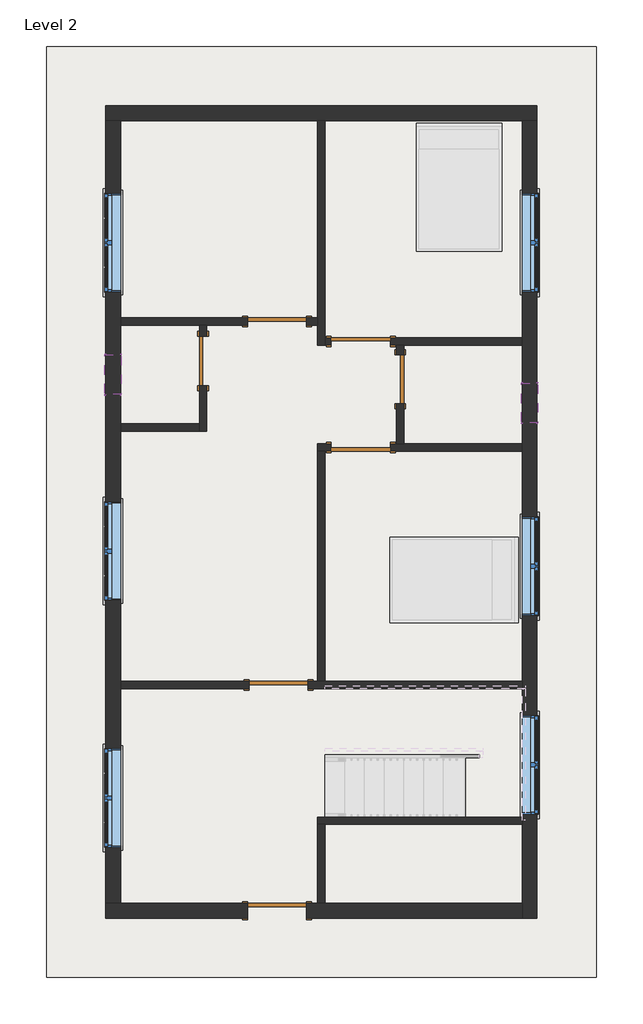
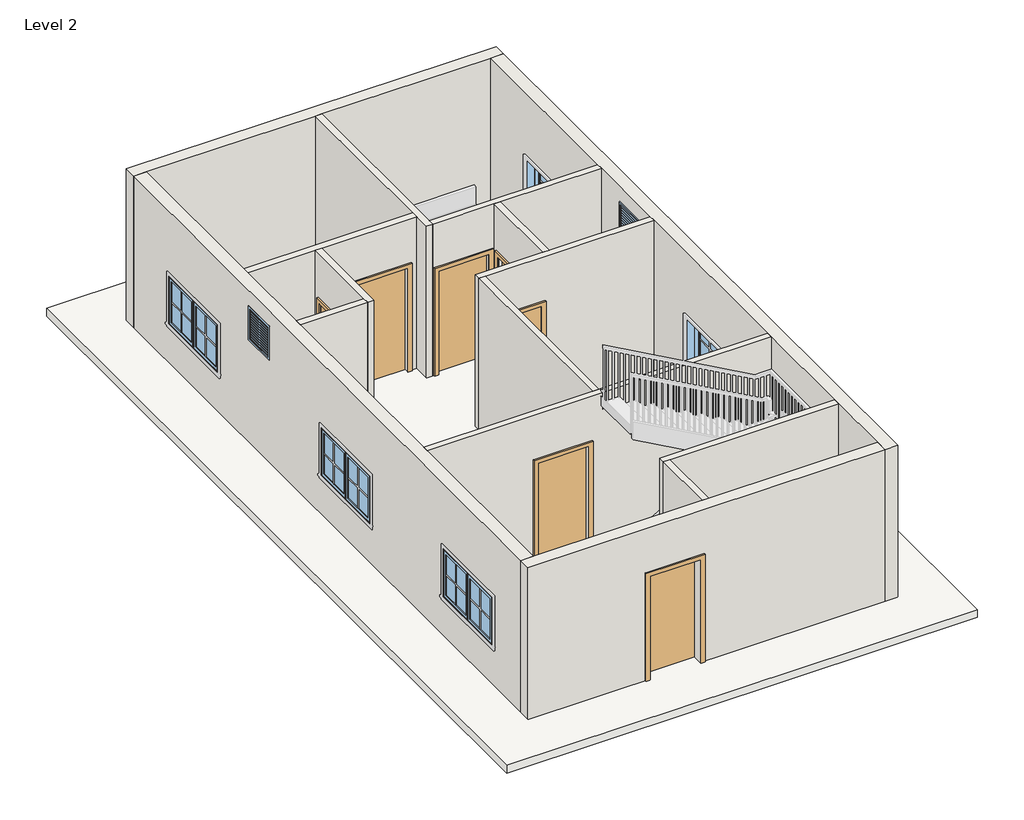
# One storey, part 1 of 3: 15 walls, 8 windows, 7 doors, 1 roof.
"""IFC4 building model written with IfcOpenShell, lengths in millimetres."""

from ifc_helpers import new_model, si_unit, frame, origin, place, context, project, spatial, polyline, outline, extrude, faceted_brep, transform, mapped, element, save
from components import door_78caadf7, door_214872d5, single_flush_door_3_e5f9f3c4, single_flush_door_3_305aa2a5, single_flush_door_3_0ca8825f, window_casement_double_win_5_c1d95f0f, window_f2d8fef0

model = new_model("IFC4")

# Units and contexts
model_context = context("Model", 3, world=origin())
ifc_project = project(units=[si_unit("LENGTHUNIT", "METRE", prefix="MILLI")], contexts=[model_context])

# Site, building, storey
site = spatial("IfcSite", under=ifc_project)
building = spatial("IfcBuilding", under=site)
storey = spatial("IfcBuildingStorey", under=building, Name="Level 2", Elevation=3048.0)

# Doors
placement = place(None, origin())
door_shape = door_78caadf7(model_context)
element("IfcDoor", 1, ObjectType="Single-Flush : 2'6\"", at=placement, inside=storey, context=model_context, shape_type="MappedRepresentation", body=[
    mapped(door_shape, transform((-35.92188, 1946.24131, 3048.0), x_axis=(0.0, 1.0, 0.0), y_axis=(-1.0, 0.0, 0.0), z_axis=(0.0, 0.0, 1.0))),
])
door_2_shape = door_214872d5(model_context)
element("IfcDoor", 2, ObjectType="Single-Flush : 2'6\"", at=placement, inside=storey, context=model_context, shape_type="MappedRepresentation", body=[
    mapped(door_2_shape, transform((-3083.92188, 2225.64131, 3048.0), x_axis=(0.0, 1.0, 0.0), y_axis=(-1.0, 0.0, 0.0), z_axis=(0.0, 0.0, 1.0))),
])
single_flush_door_3_shape = single_flush_door_3_e5f9f3c4(model_context)
element("IfcDoor", 3, ObjectType="Single-Flush : DOOR 3'", at=placement, inside=storey, context=model_context, shape_type="MappedRepresentation", body=[
    mapped(single_flush_door_3_shape, transform((-1940.92188, 2835.24131, 3048.0), x_axis=(1.0, 0.0, 0.0), y_axis=(0.0, 1.0, 0.0), z_axis=(0.0, 0.0, 1.0))),
])
element("IfcDoor", 4, ObjectType="Single-Flush : DOOR 3'", at=placement, inside=storey, context=model_context, shape_type="MappedRepresentation", body=[
    mapped(single_flush_door_3_shape, transform((-645.52188, 892.14131, 3048.0), x_axis=(-1.0, 0.0, 0.0), y_axis=(0.0, -1.0, 0.0), z_axis=(0.0, 0.0, 1.0))),
])
element("IfcDoor", 5, ObjectType="Single-Flush : DOOR 3'", at=placement, inside=storey, context=model_context, shape_type="MappedRepresentation", body=[
    mapped(single_flush_door_3_shape, transform((-1915.52188, -2778.15869, 3048.0), x_axis=(1.0, 0.0, 0.0), y_axis=(0.0, 1.0, 0.0), z_axis=(0.0, 0.0, 1.0))),
])
single_flush_door_3_2_shape = single_flush_door_3_305aa2a5(model_context)
element("IfcDoor", 6, ObjectType="Single-Flush : DOOR 3'", at=placement, inside=storey, context=model_context, shape_type="MappedRepresentation", body=[
    mapped(single_flush_door_3_2_shape, transform((-645.52188, 2530.44131, 3048.0), x_axis=(-1.0, 0.0, 0.0), y_axis=(0.0, -1.0, 0.0), z_axis=(0.0, 0.0, 1.0))),
])
single_flush_door_3_3_shape = single_flush_door_3_0ca8825f(model_context)
element("IfcDoor", 7, ObjectType="Single-Flush : DOOR 3'", at=placement, inside=storey, context=model_context, shape_type="MappedRepresentation", body=[
    mapped(single_flush_door_3_3_shape, transform((-1940.92188, -6264.30869, 3048.0), x_axis=(1.0, 0.0, 0.0), y_axis=(0.0, 1.0, 0.0), z_axis=(0.0, 0.0, 1.0))),
])

# Roof
element("IfcRoof", 8, ObjectType="ROOF 6\"", at=placement, inside=storey, context=model_context, shape_type="SweptSolid", body=[
    extrude(outline(polyline([(-5503.27188, 7083.39131), (2993.02812, 7083.39131), (2993.02812, -7293.00869), (-5503.27188, -7293.00869), (-5503.27188, 7083.39131)])), frame((0.0, 0.0, 3048.0), z_axis=(0.0, 0.0, 1.0), x_axis=(1.0, 0.0, 0.0)), (0.0, 0.0, 1.0), 152.4),
])

# Walls
element("IfcWall", 9, ObjectType="WALL 4.5'", at=placement, inside=storey, context=model_context, shape_type="Brep", body=[
    faceted_brep([(-1312.27188, 5940.39131, 3048.0), (-1312.27188, 2892.39131, 3048.0), (-1312.27188, 2778.09131, 3048.0), (-1312.27188, 2473.29131, 3048.0), (-1312.27188, 2473.29131, 6096.0), (-1312.27188, 2778.09131, 6096.0), (-1312.27188, 2892.39131, 6096.0), (-1312.27188, 5940.39131, 6096.0), (-1197.97188, 5940.39131, 3048.0), (-1197.97188, 5940.39131, 6096.0), (-1197.97188, 2587.59131, 6096.0), (-1197.97188, 2473.29131, 6096.0), (-1197.97188, 2473.29131, 3048.0), (-1197.97188, 2587.59131, 3048.0)], [[[0, 1, 2, 3, 4, 5, 6, 7]], [[8, 9, 10, 11, 12, 13]], [[3, 2, 1, 0, 8, 13, 12]], [[0, 7, 9, 8]], [[4, 3, 12, 11]], [[7, 6, 5, 4, 11, 10, 9]]]),
])
element("IfcWall", 10, ObjectType="WALL 4.5'", at=placement, inside=storey, context=model_context, shape_type="Brep", body=[
    faceted_brep([(-1197.97188, 2473.29131, 3048.0), (-1102.72188, 2473.29131, 3048.0), (-1102.72188, 2473.29131, 5181.6), (-188.32188, 2473.29131, 5181.6), (-188.32188, 2473.29131, 3048.0), (-93.07188, 2473.29131, 3048.0), (21.22812, 2473.29131, 3048.0), (1850.02812, 2473.29131, 3048.0), (1850.02812, 2473.29131, 6096.0), (21.22812, 2473.29131, 6096.0), (-93.07188, 2473.29131, 6096.0), (-1197.97188, 2473.29131, 6096.0), (-1102.72188, 2587.59131, 5181.6), (-1102.72188, 2587.59131, 3048.0), (-1197.97188, 2587.59131, 3048.0), (-1197.97188, 2587.59131, 6096.0), (1850.02812, 2587.59131, 6096.0), (1850.02812, 2587.59131, 3048.0), (-188.32188, 2587.59131, 3048.0), (-188.32188, 2587.59131, 5181.6)], [[[0, 1, 2, 3, 4, 5, 6, 7, 8, 9, 10, 11]], [[12, 13, 14, 15, 16, 17, 18, 19]], [[18, 17, 7, 6, 5, 4]], [[14, 13, 1, 0]], [[0, 11, 15, 14]], [[8, 7, 17, 16]], [[2, 1, 13, 12]], [[3, 2, 12, 19]], [[4, 3, 19, 18]], [[11, 10, 9, 8, 16, 15]]]),
])
element("IfcWall", 11, ObjectType="WALL 4.5'", at=placement, inside=storey, context=model_context, shape_type="Brep", body=[
    faceted_brep([(-1312.27188, 2892.39131, 3048.0), (-1483.72188, 2892.39131, 3048.0), (-1483.72188, 2892.39131, 5181.6), (-2398.12188, 2892.39131, 5181.6), (-2398.12188, 2892.39131, 3048.0), (-4360.27188, 2892.39131, 3048.0), (-4360.27188, 2892.39131, 6096.0), (-1312.27188, 2892.39131, 6096.0), (-1483.72188, 2778.09131, 5181.6), (-1483.72188, 2778.09131, 3048.0), (-1312.27188, 2778.09131, 3048.0), (-1312.27188, 2778.09131, 6096.0), (-3026.77188, 2778.09131, 6096.0), (-3141.07188, 2778.09131, 6096.0), (-4360.27188, 2778.09131, 6096.0), (-4360.27188, 2778.09131, 3048.0), (-3141.07188, 2778.09131, 3048.0), (-3026.77188, 2778.09131, 3048.0), (-2398.12188, 2778.09131, 3048.0), (-2398.12188, 2778.09131, 5181.6)], [[[0, 1, 2, 3, 4, 5, 6, 7]], [[8, 9, 10, 11, 12, 13, 14, 15, 16, 17, 18, 19]], [[10, 9, 1, 0]], [[18, 17, 16, 15, 5, 4]], [[6, 5, 15, 14]], [[0, 7, 11, 10]], [[2, 1, 9, 8]], [[3, 2, 8, 19]], [[4, 3, 19, 18]], [[7, 6, 14, 13, 12, 11]]]),
])
element("IfcWall", 12, ObjectType="WALL 4.5'", at=placement, inside=storey, context=model_context, shape_type="Brep", body=[
    faceted_brep([(-3141.07188, 2778.09131, 3048.0), (-3141.07188, 2606.64131, 3048.0), (-3141.07188, 2606.64131, 5181.6), (-3141.07188, 1844.64131, 5181.6), (-3141.07188, 1844.64131, 3048.0), (-3141.07188, 1254.09131, 3048.0), (-3141.07188, 1139.79131, 3048.0), (-3141.07188, 1139.79131, 6096.0), (-3141.07188, 1254.09131, 6096.0), (-3141.07188, 2778.09131, 6096.0), (-3026.77188, 2606.64131, 5181.6), (-3026.77188, 2606.64131, 3048.0), (-3026.77188, 2778.09131, 3048.0), (-3026.77188, 2778.09131, 6096.0), (-3026.77188, 1139.79131, 6096.0), (-3026.77188, 1139.79131, 3048.0), (-3026.77188, 1844.64131, 3048.0), (-3026.77188, 1844.64131, 5181.6)], [[[0, 1, 2, 3, 4, 5, 6, 7, 8, 9]], [[10, 11, 12, 13, 14, 15, 16, 17]], [[16, 15, 6, 5, 4]], [[12, 11, 1, 0]], [[0, 9, 13, 12]], [[7, 6, 15, 14]], [[2, 1, 11, 10]], [[3, 2, 10, 17]], [[4, 3, 17, 16]], [[9, 8, 7, 14, 13]]]),
])
element("IfcWall", 13, ObjectType="WALL 4.5'", at=placement, inside=storey, context=model_context, shape_type="SweptSolid", body=[
    extrude(outline(polyline([(-4360.27188, 1254.09131), (-3141.07188, 1254.09131), (-3141.07188, 1139.79131), (-4360.27188, 1139.79131), (-4360.27188, 1254.09131)])), frame((0.0, 0.0, 3048.0), z_axis=(0.0, 0.0, 1.0), x_axis=(1.0, 0.0, 0.0)), (0.0, 0.0, 1.0), 3048.0),
])
element("IfcWall", 14, ObjectType="WALL 4.5'", at=placement, inside=storey, context=model_context, shape_type="SweptSolid", body=[
    extrude(outline(polyline([(2473.29131, 3048.0), (2327.24131, 3048.0), (2327.24131, 5181.6), (1565.24131, 5181.6), (1565.24131, 3048.0), (949.29131, 3048.0), (949.29131, 6096.0), (2473.29131, 6096.0), (2473.29131, 3048.0)])), frame((-93.07188, 0.0, 0.0), z_axis=(1.0, 0.0, 0.0), x_axis=(0.0, 1.0, 0.0)), (0.0, 0.0, 1.0), 114.3),
])
element("IfcWall", 15, ObjectType="WALL 4.5'", at=placement, inside=storey, context=model_context, shape_type="Brep", body=[
    faceted_brep([(-1102.72188, 949.29131, 5181.6), (-1102.72188, 949.29131, 3048.0), (-1312.27188, 949.29131, 3048.0), (-1312.27188, 949.29131, 6096.0), (-93.07188, 949.29131, 6096.0), (21.22812, 949.29131, 6096.0), (1850.02812, 949.29131, 6096.0), (1850.02812, 949.29131, 3048.0), (21.22812, 949.29131, 3048.0), (-93.07188, 949.29131, 3048.0), (-188.32188, 949.29131, 3048.0), (-188.32188, 949.29131, 5181.6), (-1312.27188, 834.99131, 3048.0), (-1197.97188, 834.99131, 3048.0), (-1102.72188, 834.99131, 3048.0), (-1102.72188, 834.99131, 5181.6), (-188.32188, 834.99131, 5181.6), (-188.32188, 834.99131, 3048.0), (1850.02812, 834.99131, 3048.0), (1850.02812, 834.99131, 6096.0), (-1197.97188, 834.99131, 6096.0), (-1312.27188, 834.99131, 6096.0)], [[[0, 1, 2, 3, 4, 5, 6, 7, 8, 9, 10, 11]], [[12, 13, 14, 15, 16, 17, 18, 19, 20, 21]], [[2, 1, 14, 13, 12]], [[10, 9, 8, 7, 18, 17]], [[7, 6, 19, 18]], [[3, 2, 12, 21]], [[15, 14, 1, 0]], [[16, 15, 0, 11]], [[17, 16, 11, 10]], [[6, 5, 4, 3, 21, 20, 19]]]),
])
element("IfcWall", 16, ObjectType="WALL 4.5'", at=placement, inside=storey, context=model_context, shape_type="SweptSolid", body=[
    extrude(outline(polyline([(-1312.27188, -2721.00869), (-1312.27188, 834.99131), (-1197.97188, 834.99131), (-1197.97188, -2721.00869), (-1312.27188, -2721.00869)])), frame((0.0, 0.0, 3048.0), z_axis=(0.0, 0.0, 1.0), x_axis=(1.0, 0.0, 0.0)), (0.0, 0.0, 1.0), 3048.0),
])
element("IfcWall", 17, ObjectType="WALL 4.5'", at=placement, inside=storey, context=model_context, shape_type="Brep", body=[
    faceted_brep([(1850.02812, -2721.00869, 3048.0), (-1197.97188, -2721.00869, 3048.0), (-1312.27188, -2721.00869, 3048.0), (-1458.32188, -2721.00869, 3048.0), (-1458.32188, -2721.00869, 5181.6), (-2372.72188, -2721.00869, 5181.6), (-2372.72188, -2721.00869, 3048.0), (-4360.27188, -2721.00869, 3048.0), (-4360.27188, -2721.00869, 6096.0), (-1312.27188, -2721.00869, 6096.0), (-1197.97188, -2721.00869, 6096.0), (1850.02812, -2721.00869, 6096.0), (-1458.32188, -2835.30869, 5181.6), (-1458.32188, -2835.30869, 3048.0), (1850.02812, -2835.30869, 3048.0), (1850.02812, -2835.30869, 6096.0), (-4360.27188, -2835.30869, 6096.0), (-4360.27188, -2835.30869, 3048.0), (-2372.72188, -2835.30869, 3048.0), (-2372.72188, -2835.30869, 5181.6)], [[[0, 1, 2, 3, 4, 5, 6, 7, 8, 9, 10, 11]], [[12, 13, 14, 15, 16, 17, 18, 19]], [[18, 17, 7, 6]], [[14, 13, 3, 2, 1, 0]], [[0, 11, 15, 14]], [[8, 7, 17, 16]], [[4, 3, 13, 12]], [[5, 4, 12, 19]], [[6, 5, 19, 18]], [[11, 10, 9, 8, 16, 15]]]),
])
element("IfcWall", 18, ObjectType="WALL 4.5'", at=placement, inside=storey, context=model_context, shape_type="Brep", body=[
    faceted_brep([(1850.02812, -4816.50869, 3048.0), (-1312.27188, -4816.50869, 3048.0), (-1312.27188, -4816.50869, 6096.0), (1850.02812, -4816.50869, 6096.0), (1850.02812, -4930.80869, 3048.0), (1850.02812, -4930.80869, 6096.0), (-1197.97188, -4930.80869, 6096.0), (-1312.27188, -4930.80869, 6096.0), (-1312.27188, -4930.80869, 3048.0), (-1197.97188, -4930.80869, 3048.0)], [[[0, 1, 2, 3]], [[4, 5, 6, 7, 8, 9]], [[1, 0, 4, 9, 8]], [[0, 3, 5, 4]], [[2, 1, 8, 7]], [[3, 2, 7, 6, 5]]]),
])
element("IfcWall", 19, ObjectType="WALL 4.5'", at=placement, inside=storey, context=model_context, shape_type="SweptSolid", body=[
    extrude(outline(polyline([(-1312.27188, -6150.00869), (-1312.27188, -4930.80869), (-1197.97188, -4930.80869), (-1197.97188, -6150.00869), (-1312.27188, -6150.00869)])), frame((0.0, 0.0, 3048.0), z_axis=(0.0, 0.0, 1.0), x_axis=(1.0, 0.0, 0.0)), (0.0, 0.0, 1.0), 3048.0),
])
element("IfcWall", 20, ObjectType="WALL 9\"", at=placement, inside=storey, context=model_context, shape_type="Brep", body=[
    faceted_brep([(-4588.87188, 5940.39131, 3048.0), (-4360.27188, 5940.39131, 3048.0), (-1312.27188, 5940.39131, 3048.0), (-1197.97188, 5940.39131, 3048.0), (1850.02812, 5940.39131, 3048.0), (2078.62812, 5940.39131, 3048.0), (2078.62812, 5940.39131, 6096.0), (1850.02812, 5940.39131, 6096.0), (-1197.97188, 5940.39131, 6096.0), (-1312.27188, 5940.39131, 6096.0), (-4360.27188, 5940.39131, 6096.0), (-4588.87188, 5940.39131, 6096.0), (-4588.87188, 6168.99131, 3048.0), (-4588.87188, 6168.99131, 6096.0), (2078.62812, 6168.99131, 6096.0), (2078.62812, 6168.99131, 3048.0)], [[[0, 1, 2, 3, 4, 5, 6, 7, 8, 9, 10, 11]], [[12, 13, 14, 15]], [[5, 4, 3, 2, 1, 0, 12, 15]], [[6, 5, 15, 14]], [[0, 11, 13, 12]], [[11, 10, 9, 8, 7, 6, 14, 13]]]),
])
element("IfcWall", 21, ObjectType="WALL 9\"", at=placement, inside=storey, context=model_context, shape_type="Brep", body=[
    faceted_brep([(1850.02812, 5940.39131, 3048.0), (1850.02812, 2587.59131, 3048.0), (1850.02812, 2473.29131, 3048.0), (1850.02812, 949.29131, 3048.0), (1850.02812, 834.99131, 3048.0), (1850.02812, -2721.00869, 3048.0), (1850.02812, -2835.30869, 3048.0), (1850.02812, -4816.50869, 3048.0), (1850.02812, -4930.80869, 3048.0), (1850.02812, -6150.00869, 3048.0), (1850.02812, -6378.60869, 3048.0), (1850.02812, -6378.60869, 6096.0), (1850.02812, -6150.00869, 6096.0), (1850.02812, -4930.80869, 6096.0), (1850.02812, -4816.50869, 6096.0), (1850.02812, -2835.30869, 6096.0), (1850.02812, -2721.00869, 6096.0), (1850.02812, 834.99131, 6096.0), (1850.02812, 949.29131, 6096.0), (1850.02812, 2473.29131, 6096.0), (1850.02812, 2587.59131, 6096.0), (1850.02812, 5940.39131, 6096.0), (1850.02812, -4772.05869, 4876.8), (1850.02812, -4772.05869, 3962.4), (1850.02812, -3248.05869, 3962.4), (1850.02812, -3248.05869, 4876.8), (1850.02812, 3292.44131, 4876.8), (1850.02812, 3292.44131, 3962.4), (1850.02812, 4816.44131, 3962.4), (1850.02812, 4816.44131, 4876.8), (1850.02812, -1705.00869, 4876.8), (1850.02812, -1705.00869, 3962.4), (1850.02812, -181.00869, 3962.4), (1850.02812, -181.00869, 4876.8), (1850.02812, 1273.14131, 5791.2), (1850.02812, 1273.14131, 5181.6), (1850.02812, 1882.74131, 5181.6), (1850.02812, 1882.74131, 5791.2), (2078.62812, 5940.39131, 3048.0), (2078.62812, 5940.39131, 6096.0), (2078.62812, -6378.60869, 6096.0), (2078.62812, -6378.60869, 3048.0), (2078.62812, -4772.05869, 4876.8), (2078.62812, -3248.05869, 4876.8), (2078.62812, -3248.05869, 3962.4), (2078.62812, -4772.05869, 3962.4), (2078.62812, 3292.44131, 4876.8), (2078.62812, 4816.44131, 4876.8), (2078.62812, 4816.44131, 3962.4), (2078.62812, 3292.44131, 3962.4), (2078.62812, -1705.00869, 4876.8), (2078.62812, -181.00869, 4876.8), (2078.62812, -181.00869, 3962.4), (2078.62812, -1705.00869, 3962.4), (2078.62812, 1273.14131, 5791.2), (2078.62812, 1882.74131, 5791.2), (2078.62812, 1882.74131, 5181.6), (2078.62812, 1273.14131, 5181.6)], [[[0, 1, 2, 3, 4, 5, 6, 7, 8, 9, 10, 11, 12, 13, 14, 15, 16, 17, 18, 19, 20, 21], [22, 23, 24, 25], [26, 27, 28, 29], [30, 31, 32, 33], [34, 35, 36, 37]], [[38, 39, 40, 41], [42, 43, 44, 45], [46, 47, 48, 49], [50, 51, 52, 53], [54, 55, 56, 57]], [[10, 9, 8, 7, 6, 5, 4, 3, 2, 1, 0, 38, 41]], [[0, 21, 39, 38]], [[11, 10, 41, 40]], [[23, 22, 42, 45]], [[24, 23, 45, 44]], [[25, 24, 44, 43]], [[22, 25, 43, 42]], [[27, 26, 46, 49]], [[28, 27, 49, 48]], [[29, 28, 48, 47]], [[26, 29, 47, 46]], [[31, 30, 50, 53]], [[32, 31, 53, 52]], [[33, 32, 52, 51]], [[30, 33, 51, 50]], [[35, 34, 54, 57]], [[36, 35, 57, 56]], [[37, 36, 56, 55]], [[34, 37, 55, 54]], [[21, 20, 19, 18, 17, 16, 15, 14, 13, 12, 11, 40, 39]]]),
])
element("IfcWall", 22, ObjectType="WALL 9\"", at=placement, inside=storey, context=model_context, shape_type="Brep", body=[
    faceted_brep([(1850.02812, -6150.00869, 3048.0), (-1197.97188, -6150.00869, 3048.0), (-1312.27188, -6150.00869, 3048.0), (-1483.72188, -6150.00869, 3048.0), (-1483.72188, -6150.00869, 5181.6), (-2398.12188, -6150.00869, 5181.6), (-2398.12188, -6150.00869, 3048.0), (-4360.27188, -6150.00869, 3048.0), (-4588.87188, -6150.00869, 3048.0), (-4588.87188, -6150.00869, 6096.0), (-4360.27188, -6150.00869, 6096.0), (-1312.27188, -6150.00869, 6096.0), (-1197.97188, -6150.00869, 6096.0), (1850.02812, -6150.00869, 6096.0), (-1483.72188, -6378.60869, 5181.6), (-1483.72188, -6378.60869, 3048.0), (1850.02812, -6378.60869, 3048.0), (1850.02812, -6378.60869, 6096.0), (-4588.87188, -6378.60869, 6096.0), (-4588.87188, -6378.60869, 3048.0), (-2398.12188, -6378.60869, 3048.0), (-2398.12188, -6378.60869, 5181.6)], [[[0, 1, 2, 3, 4, 5, 6, 7, 8, 9, 10, 11, 12, 13]], [[14, 15, 16, 17, 18, 19, 20, 21]], [[20, 19, 8, 7, 6]], [[16, 15, 3, 2, 1, 0]], [[0, 13, 17, 16]], [[9, 8, 19, 18]], [[4, 3, 15, 14]], [[5, 4, 14, 21]], [[6, 5, 21, 20]], [[13, 12, 11, 10, 9, 18, 17]]]),
])
element("IfcWall", 23, ObjectType="WALL 9\"", at=placement, inside=storey, context=model_context, shape_type="Brep", body=[
    faceted_brep([(-4360.27188, -6150.00869, 3048.0), (-4360.27188, -2835.30869, 3048.0), (-4360.27188, -2721.00869, 3048.0), (-4360.27188, 1139.79131, 3048.0), (-4360.27188, 1254.09131, 3048.0), (-4360.27188, 2778.09131, 3048.0), (-4360.27188, 2892.39131, 3048.0), (-4360.27188, 5940.39131, 3048.0), (-4360.27188, 5940.39131, 6096.0), (-4360.27188, 2892.39131, 6096.0), (-4360.27188, 2778.09131, 6096.0), (-4360.27188, 1254.09131, 6096.0), (-4360.27188, 1139.79131, 6096.0), (-4360.27188, -2721.00869, 6096.0), (-4360.27188, -2835.30869, 6096.0), (-4360.27188, -6150.00869, 6096.0), (-4360.27188, 4816.44131, 4876.8), (-4360.27188, 4816.44131, 3962.4), (-4360.27188, 3292.44131, 3962.4), (-4360.27188, 3292.44131, 4876.8), (-4360.27188, 53.94131, 4876.8), (-4360.27188, 53.94131, 3962.4), (-4360.27188, -1470.05869, 3962.4), (-4360.27188, -1470.05869, 4876.8), (-4360.27188, -3759.23369, 4876.8), (-4360.27188, -3759.23369, 3962.4), (-4360.27188, -5283.23369, 3962.4), (-4360.27188, -5283.23369, 4876.8), (-4360.27188, 1711.29131, 5791.2), (-4360.27188, 2320.89131, 5791.2), (-4360.27188, 2320.89131, 5181.6), (-4360.27188, 1711.29131, 5181.6), (-4588.87188, -6150.00869, 3048.0), (-4588.87188, -6150.00869, 6096.0), (-4588.87188, 5940.39131, 6096.0), (-4588.87188, 5940.39131, 3048.0), (-4588.87188, 4816.44131, 4876.8), (-4588.87188, 3292.44131, 4876.8), (-4588.87188, 3292.44131, 3962.4), (-4588.87188, 4816.44131, 3962.4), (-4588.87188, 53.94131, 4876.8), (-4588.87188, -1470.05869, 4876.8), (-4588.87188, -1470.05869, 3962.4), (-4588.87188, 53.94131, 3962.4), (-4588.87188, -3759.23369, 4876.8), (-4588.87188, -5283.23369, 4876.8), (-4588.87188, -5283.23369, 3962.4), (-4588.87188, -3759.23369, 3962.4), (-4588.87188, 1711.29131, 5791.2), (-4588.87188, 1711.29131, 5181.6), (-4588.87188, 2320.89131, 5181.6), (-4588.87188, 2320.89131, 5791.2)], [[[0, 1, 2, 3, 4, 5, 6, 7, 8, 9, 10, 11, 12, 13, 14, 15], [16, 17, 18, 19], [20, 21, 22, 23], [24, 25, 26, 27], [28, 29, 30, 31]], [[32, 33, 34, 35], [36, 37, 38, 39], [40, 41, 42, 43], [44, 45, 46, 47], [48, 49, 50, 51]], [[7, 6, 5, 4, 3, 2, 1, 0, 32, 35]], [[8, 7, 35, 34]], [[0, 15, 33, 32]], [[17, 16, 36, 39]], [[18, 17, 39, 38]], [[19, 18, 38, 37]], [[16, 19, 37, 36]], [[21, 20, 40, 43]], [[22, 21, 43, 42]], [[23, 22, 42, 41]], [[20, 23, 41, 40]], [[25, 24, 44, 47]], [[26, 25, 47, 46]], [[27, 26, 46, 45]], [[24, 27, 45, 44]], [[49, 48, 28, 31]], [[50, 49, 31, 30]], [[51, 50, 30, 29]], [[48, 51, 29, 28]], [[15, 14, 13, 12, 11, 10, 9, 8, 34, 33]]]),
])

# Windows
window_casement_double_win_5_shape = window_casement_double_win_5_c1d95f0f(model_context)
element("IfcWindow", 24, ObjectType="Window-Casement-Double : WIN 5'", at=placement, inside=storey, context=model_context, shape_type="MappedRepresentation", body=[
    mapped(window_casement_double_win_5_shape, transform((-4474.57188, 4054.44131, 3048.0), x_axis=(0.0, 1.0, 0.0), y_axis=(-1.0, 0.0, 0.0), z_axis=(0.0, 0.0, 1.0))),
])
element("IfcWindow", 25, ObjectType="Window-Casement-Double : WIN 5'", at=placement, inside=storey, context=model_context, shape_type="MappedRepresentation", body=[
    mapped(window_casement_double_win_5_shape, transform((-4474.57188, -708.05869, 3048.0), x_axis=(0.0, 1.0, 0.0), y_axis=(-1.0, 0.0, 0.0), z_axis=(0.0, 0.0, 1.0))),
])
element("IfcWindow", 26, ObjectType="Window-Casement-Double : WIN 5'", at=placement, inside=storey, context=model_context, shape_type="MappedRepresentation", body=[
    mapped(window_casement_double_win_5_shape, transform((-4474.57188, -4521.23369, 3048.0), x_axis=(0.0, 1.0, 0.0), y_axis=(-1.0, 0.0, 0.0), z_axis=(0.0, 0.0, 1.0))),
])
element("IfcWindow", 27, ObjectType="Window-Casement-Double : WIN 5'", at=placement, inside=storey, context=model_context, shape_type="MappedRepresentation", body=[
    mapped(window_casement_double_win_5_shape, transform((1964.32812, -4010.05869, 3048.0), x_axis=(0.0, -1.0, 0.0), y_axis=(1.0, 0.0, 0.0), z_axis=(0.0, 0.0, 1.0))),
])
element("IfcWindow", 28, ObjectType="Window-Casement-Double : WIN 5'", at=placement, inside=storey, context=model_context, shape_type="MappedRepresentation", body=[
    mapped(window_casement_double_win_5_shape, transform((1964.32812, 4054.44131, 3048.0), x_axis=(0.0, -1.0, 0.0), y_axis=(1.0, 0.0, 0.0), z_axis=(0.0, 0.0, 1.0))),
])
element("IfcWindow", 29, ObjectType="Window-Casement-Double : WIN 5'", at=placement, inside=storey, context=model_context, shape_type="MappedRepresentation", body=[
    mapped(window_casement_double_win_5_shape, transform((1964.32812, -943.00869, 3048.0), x_axis=(0.0, -1.0, 0.0), y_axis=(1.0, 0.0, 0.0), z_axis=(0.0, 0.0, 1.0))),
])
window_shape = window_f2d8fef0(model_context)
element("IfcWindow", 30, ObjectType="Window-Louvers : 24\" x 24\"", at=placement, inside=storey, context=model_context, shape_type="MappedRepresentation", body=[
    mapped(window_shape, transform((1957.97812, 1577.94131, 4267.2), x_axis=(0.0, 1.0, 0.0), y_axis=(-1.0, 0.0, 0.0), z_axis=(0.0, 0.0, 1.0))),
])
element("IfcWindow", 31, ObjectType="Window-Louvers : 24\" x 24\"", at=placement, inside=storey, context=model_context, shape_type="MappedRepresentation", body=[
    mapped(window_shape, transform((-4480.92188, 2016.09131, 4267.2), x_axis=(0.0, 1.0, 0.0), y_axis=(-1.0, 0.0, 0.0), z_axis=(0.0, 0.0, 1.0))),
])

save(model, "model.ifc")

# Revit data of these elements
# Type "Single-Flush : 2'6\""
#   Type Mark = "9"
#   Construction Type Id = "MDOOR"
#   Assembly Code = "C1020"
#   Analytic Construction = "Metal"
#   Thickness = 0' - 2"
#   Heat Transfer Coefficient (U) = 0.651978 BTU/(h·ft²·°F)
#   Height = 7' - 0"
#   Trim Projection Ext = 0' - 1"
#   Trim Projection Int = 0' - 1"
#   Trim Width = 0' - 3"
#   Width = 2' - 6"
#   Define Thermal Properties by = 1
#   Door Material = Door - Panel
#   Frame Material = Door - Frame
#   Visual Light Transmittance = 0
#   Solar Heat Gain Coefficient = 0
#   Function = (empty or 0)
#   Wall Closure = (empty or 0)
# Type "Single-Flush : DOOR 3'"
#   Type Mark = "8"
#   Construction Type Id = "MDOOR"
#   Assembly Code = "C1020"
#   Analytic Construction = "Metal"
#   Thickness = 0' - 2"
#   Heat Transfer Coefficient (U) = 0.651978 BTU/(h·ft²·°F)
#   Height = 7' - 0"
#   Trim Projection Ext = 0' - 1"
#   Trim Projection Int = 0' - 1"
#   Trim Width = 0' - 3"
#   Width = 3' - 0"
#   Define Thermal Properties by = 1
#   Door Material = Door - Panel
#   Frame Material = Door - Frame
#   Visual Light Transmittance = 0
#   Solar Heat Gain Coefficient = 0
#   Function = (empty or 0)
#   Wall Closure = (empty or 0)
# Type "ROOF 6\""
#   Assembly Code = "B1020"
#   Layers, outside or top first: 0' - 6" no material (function 1)
# Type "WALL 4.5'"
#   Assembly Code = "B2010"
#   Layers, outside or top first: 0' - 4 1/2" no material (function 1)
# Type "WALL 9\""
#   Assembly Code = "B2010"
#   Layers, outside or top first: 0' - 9" no material (function 1)
# Type "Window-Casement-Double : WIN 5'"
#   Type Mark = "18"
#   Fire Rating = "0.5h"
#   Assembly Code = "B2020100"
#   Analytic Construction = "Double glazing - domestic"
#   Frame Extension [instance default] = 0' - 0 1/4"
#   Window Inset [instance default] = 0' - 0"
#   Wall Thickness [instance default] = 0' - 6"
#   Interior Wall Closure [instance default] = 0' - 2 1/4"
#   Half Width = 2' - 6"
#   Visual Light Transmittance = 0.81
#   Thermal Resistance (R) = 1.8146 (h·ft²·°F)/BTU
#   Solar Heat Gain Coefficient = 0.76
#   Rough Width = 5' - 0 1/2"
#   Rough Height = 3' - 0 1/2"
#   Height = 3' - 0"
#   Heat Transfer Coefficient (U) = 0.5511 BTU/(h·ft²·°F)
#   Exterior Wall Closure [instance default] = 0' - 1 1/4"
#   Extension Jamb [instance default] = 0' - 2 1/4"
#   Default Sill Height = 3' - 0"
#   Width = 5' - 0"
#   Muntin Visibility = yes
#   Interior Trim Visibility [instance default] = yes
#   Exterior Trim Visibility [instance default] = yes
#   Extension Jamb Visibility [instance default] = yes
#   Interior Trim Material = Wood - Stained
#   Muntin Pattern = Muntin Pattern_2x2 : Muntin Pattern_2x2
#   Interior Trim = Trim-Window-Interior-Flat : Picture Frame
#   Interior Frame Material = Wood - Stained
#   Glass Panel Material = Glass
#   Exterior Trim Material = Clad - White
#   Exterior Trim = Trim-Window-Exterior-Flat : with Sill
#   Exterior Frame Material = Clad - White
#   Wall Closure = (empty or 0)
# Type "Window-Louvers : 24\" x 24\""
#   Type Mark = "19"
#   Construction Type Id = "GSP4R"
#   Assembly Code = "B20"
#   Analytic Construction = "1/8 in Pilkington single glazing"
#   Visual Light Transmittance = 0.9
#   Thermal Resistance (R) = 1.53941 (h·ft²·°F)/BTU
#   Solar Heat Gain Coefficient = 0.78
#   Max Height = 1' - 11.74264"
#   Height = 2' - 0"
#   Heat Transfer Coefficient (U) = 0.6496 BTU/(h·ft²·°F)
#   Blade Width [instance default] = 1' - 10 1/2"
#   Blade Vertical Thickness = 0' - 0.35355"
#   Blade Thickness = 0' - 0 1/4"
#   Blade Spacing = 0' - 1 1/2"
#   Blade Height = 0' - 1.85355"
#   Blade Depth = 0' - 3"
#   Blade Angle = 45.00°
#   Default Sill Height = 3' - 0"
#   Trim Projection_Exterior = 0' - 0 1/2"
#   Trim Projection_Interior = 0' - 0 1/2"
#   Trim Width_Exterior = 0' - 1 1/2"
#   Trim Width_Interior = 0' - 1 1/2"
#   Width = 2' - 0"
#   Max Blade Count = 12
#   Define Thermal Properties by = 1
#   Blade Count = 12
#   Frame Material = Birch
#   Louver Material = Birch
#   Trim Exterior Material = Birch
#   Trim Interior Material = Birch
#   Wall Closure = (empty or 0)
# Elements 1, 2 (IfcDoor, "Single-Flush : 2'6\"")
#   Phase Created = New Construction
#   Materials on its faces: "Door - Frame", "Door - Panel"
# Elements 3, 4, 5, 6, 7 (IfcDoor, "Single-Flush : DOOR 3'")
#   Phase Created = New Construction
#   Materials on its faces: "Door - Frame", "Door - Panel"
# Element 8 (IfcRoof, "ROOF 6\"")
#   built-in parameter 1001705 = 10.5 (stored number, unit not read)
#   built-in parameter 1001710 = 33615
#   Phase Created = New Construction
#   Materials on its faces: "Parking Stripe", "Default Roof", "Wood - Stained"
# Elements 9, 10, 11, 12, 13, 14, 15, 16, 17, 18, 19 (IfcWall, "WALL 4.5'")
#   Top Offset = 0' - 0"
#   Base Offset = 0' - 0"
#   Unconnected Height = 10' - 0"
#   wall height = 10' - 0"
#   Phase Created = New Construction
#   Base Constraint = Level 2
#   Materials on its faces: "Default Wall"
# Elements 20, 21, 22, 23 (IfcWall, "WALL 9\"")
#   Top Offset = 0' - 0"
#   Base Offset = 0' - 0"
#   Unconnected Height = 10' - 0"
#   wall height = 10' - 0"
#   Phase Created = New Construction
#   Base Constraint = Level 2
#   Materials on its faces: "Default Wall", "Copper"
# Element 24 (IfcWindow, "Window-Casement-Double : WIN 5'")
#   Mark = "9"
#   Window Inset = 0' - 0"
#   Interior Wall Closure = 0' - 2 1/4"
#   Frame Extension = 0' - 0 1/4"
#   Exterior Wall Closure = 0' - 1 1/4"
#   Interior Trim Visibility = yes
#   Exterior Trim Visibility = yes
#   Phase Created = New Construction
#   Materials on its faces: "Wood - Stained", "Glass", "Clad - White"
# Element 25 (IfcWindow, "Window-Casement-Double : WIN 5'")
#   Mark = "10"
#   Window Inset = 0' - 0"
#   Interior Wall Closure = 0' - 2 1/4"
#   Frame Extension = 0' - 0 1/4"
#   Exterior Wall Closure = 0' - 1 1/4"
#   Interior Trim Visibility = yes
#   Exterior Trim Visibility = yes
#   Phase Created = New Construction
#   Materials on its faces: "Wood - Stained", "Glass", "Clad - White"
# Element 26 (IfcWindow, "Window-Casement-Double : WIN 5'")
#   Mark = "11"
#   Window Inset = 0' - 0"
#   Interior Wall Closure = 0' - 2 1/4"
#   Frame Extension = 0' - 0 1/4"
#   Exterior Wall Closure = 0' - 1 1/4"
#   Interior Trim Visibility = yes
#   Exterior Trim Visibility = yes
#   Phase Created = New Construction
#   Materials on its faces: "Wood - Stained", "Glass", "Clad - White"
# Element 27 (IfcWindow, "Window-Casement-Double : WIN 5'")
#   Mark = "12"
#   Window Inset = 0' - 0"
#   Interior Wall Closure = 0' - 2 1/4"
#   Frame Extension = 0' - 0 1/4"
#   Exterior Wall Closure = 0' - 1 1/4"
#   Interior Trim Visibility = yes
#   Exterior Trim Visibility = yes
#   Phase Created = New Construction
#   Materials on its faces: "Wood - Stained", "Glass", "Clad - White"
# Element 28 (IfcWindow, "Window-Casement-Double : WIN 5'")
#   Mark = "13"
#   Window Inset = 0' - 0"
#   Interior Wall Closure = 0' - 2 1/4"
#   Frame Extension = 0' - 0 1/4"
#   Exterior Wall Closure = 0' - 1 1/4"
#   Interior Trim Visibility = yes
#   Exterior Trim Visibility = yes
#   Phase Created = New Construction
#   Materials on its faces: "Wood - Stained", "Glass", "Clad - White"
# Element 29 (IfcWindow, "Window-Casement-Double : WIN 5'")
#   Mark = "14"
#   Window Inset = 0' - 0"
#   Interior Wall Closure = 0' - 2 1/4"
#   Frame Extension = 0' - 0 1/4"
#   Exterior Wall Closure = 0' - 1 1/4"
#   Interior Trim Visibility = yes
#   Exterior Trim Visibility = yes
#   Phase Created = New Construction
#   Materials on its faces: "Wood - Stained", "Glass", "Clad - White"
# Element 30 (IfcWindow, "Window-Louvers : 24\" x 24\"")
#   Mark = "15"
#   Blade Width = 1' - 10 1/2"
#   Phase Created = New Construction
#   Materials on its faces: "Birch"
# Element 31 (IfcWindow, "Window-Louvers : 24\" x 24\"")
#   Mark = "16"
#   Blade Width = 1' - 10 1/2"
#   Phase Created = New Construction
#   Materials on its faces: "Birch"
# Materials
#   "Door - Panel": class "Wood", colour RGB 210 159 95, transparency 0, Cost = 0
#   "Door - Frame": colour RGB 118 70 51, transparency 0, Cost = 0
#   "Wood - Stained": class "Wood", colour RGB 224 178 126, transparency 0, Cost = 0
#   "Glass": class "Glass", colour RGB 0 128 192, transparency 0.75, Description = "Soda Lime Glass", Cost = 0
#   "Clad - White": class "Wood", colour RGB 242 242 238, transparency 0, Cost = 0
#   "Birch": class "Wood", colour RGB 224 178 126, transparency 0, Description = "Betula Alleghaniensis", Cost = 0
#   "Parking Stripe": class "Paint", colour RGB 250 250 91, transparency 0, Cost = 0
#   "Default Roof": colour RGB 88 101 114, transparency 0, Cost = 0
#   "Default Wall": colour RGB 128 128 128, transparency 0, Cost = 0
#   "Copper": class "Metal", colour RGB 0 0 0, transparency 0, Description = "Copper, matte finish", Cost = 0
